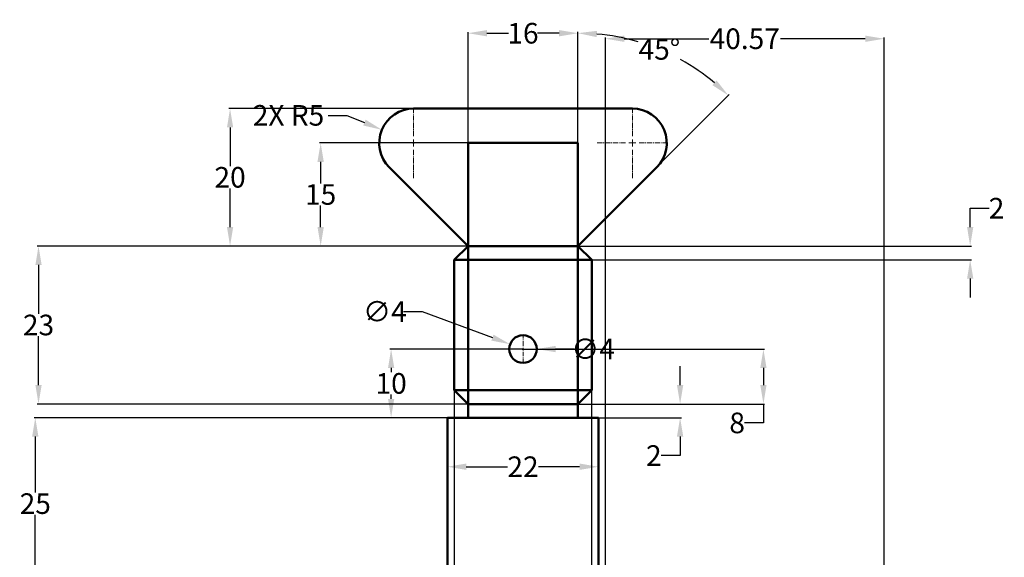
# Model space of a CAD drawing. Units: inches. Extents: x 7239 to 7401, y 3529 to 3727.
# Tile 2 of 2: x 7258 to 7401, y 3648 to 3727. Entities that reach past the tile are written whole.
import ezdxf

# ---------------------------------------------------------------- set-up
doc = ezdxf.new("R2010")
doc.units = ezdxf.units.IN
doc.header["$MEASUREMENT"] = 0
doc.linetypes.add('CENTER2', pattern=[1.125, 0.75, -0.125, 0.125, -0.125])
for name, color, linetype, lineweight in [('M-CNTR', 4, 'CENTER2', 18), ('M-DIMS', 2, 'Continuous', 25), ('M-OUTL', 7, 'Continuous', 50)]:
    doc.layers.add(name, color=color, linetype=linetype, lineweight=lineweight)
doc.styles.get("Standard").update_dxf_attribs({"font": 'arial.ttf'})
doc.dimstyles.get("Standard").update_dxf_attribs({"dimtxt": 3, "dimasz": 2.75, "dimexe": 0.18, "dimexo": 0.0625, "dimgap": 0.09, "dimtad": 0, "dimtih": 1, "dimtoh": 1, "dimdec": 0, "dimzin": 0, "dimdsep": 46, "dimtxsty": 'Standard', "dimcen": 0.09, "dimadec": 0, "dimazin": 0, "dimtfac": 1, "dimtdec": 0, "dimtofl": 0, "dimtmove": 0, "dimatfit": 3, "dimfxl": 1, "dimtolj": 1, "dimtzin": 0, "dimarcsym": 0})

# ---------------------------------------------------------------- blocks, each defined once
blk = doc.blocks.new('*U2')
at = {"layer": 'M-CNTR', "color": 0, "transparency": 16777216}
for p, q in [((0, 1), (0, 5.12)), ((-5.12, 0), (-1, 0)), ((1, 0), (5.12, 0)), ((0, -5.12), (0, -1))]:
    blk.add_line(p, q, dxfattribs=at)
at = {"layer": 'M-CNTR', "color": 0, "linetype": 'Continuous', "transparency": 16777216}
for p, q in [((-0.5, 0), (0.5, 0)), ((0, -0.5), (0, 0.5))]:
    blk.add_line(p, q, dxfattribs=at)
blk = doc.blocks.new('*U3')
at = {"layer": 'M-CNTR', "color": 0, "transparency": 16777216}
for p, q in [((0, 1), (0, 5.12)), ((-5.12, 0), (-1, 0)), ((1, 0), (5.12, 0)), ((0, -5.12), (0, -1))]:
    blk.add_line(p, q, dxfattribs=at)
at = {"layer": 'M-CNTR', "color": 0, "linetype": 'Continuous', "transparency": 16777216}
for p, q in [((-0.5, 0), (0.5, 0)), ((0, -0.5), (0, 0.5))]:
    blk.add_line(p, q, dxfattribs=at)
blk = doc.blocks.new('*U4')
at = {"layer": 'M-CNTR', "color": 0, "transparency": 16777216}
for p, q in [((0, 0.4), (0, 2.12)), ((-2.12, 0), (-0.4, 0)), ((0.4, 0), (2.12, 0)), ((0, -2.12), (0, -0.4))]:
    blk.add_line(p, q, dxfattribs=at)
at = {"layer": 'M-CNTR', "color": 0, "linetype": 'Continuous', "transparency": 16777216}
for p, q in [((-0.2, 0), (0.2, 0)), ((0, -0.2), (0, 0.2))]:
    blk.add_line(p, q, dxfattribs=at)
blk = doc.blocks.new('*D21')
at = {"layer": 'Defpoints', "color": 0, "transparency": 16777216}
for p in [(7320.11, 3668.7), (7342.11, 3668.7), (7342.11, 3661.57)]:
    blk.add_point(p, dxfattribs=at)
at = {"layer": 'M-DIMS', "color": 0, "lineweight": -2, "transparency": 16777216}
for p, q in [((7320.11, 3668.64), (7320.11, 3661.39)), ((7342.11, 3668.64), (7342.11, 3661.39)), ((7322.86, 3661.57), (7328.87, 3661.57)), ((7339.36, 3661.57), (7333.36, 3661.57))]:
    blk.add_line(p, q, dxfattribs=at)
at = {"layer": 'M-DIMS', "color": 0, "transparency": 16777216}
for points in [[(7322.86, 3662.03), (7322.86, 3661.11), (7320.11, 3661.57)], [(7339.36, 3662.03), (7339.36, 3661.11), (7342.11, 3661.57)]]:
    blk.add_solid(points, dxfattribs=at)
at = {"layer": 'M-DIMS', "color": 0, "transparency": 16777216, "insert": (7331.11, 3661.57), "char_height": 3, "attachment_point": 5}
blk.add_mtext('\\A1;22', dxfattribs=at)
blk = doc.blocks.new('*D22')
at = {"layer": 'Defpoints', "color": 0, "transparency": 16777216}
for p in [(7260.1, 3668.7), (7320.11, 3668.7), (7320.11, 3643.7)]:
    blk.add_point(p, dxfattribs=at)
at = {"layer": 'M-DIMS', "color": 0, "lineweight": -2, "transparency": 16777216}
for p, q in [((7320.05, 3668.7), (7259.92, 3668.7)), ((7260.1, 3665.95), (7260.1, 3657.82)), ((7260.1, 3646.45), (7260.1, 3654.58)), ((7320.05, 3643.7), (7259.92, 3643.7))]:
    blk.add_line(p, q, dxfattribs=at)
at = {"layer": 'M-DIMS', "color": 0, "transparency": 16777216}
for points in [[(7259.64, 3665.95), (7260.56, 3665.95), (7260.1, 3668.7)], [(7259.64, 3646.45), (7260.56, 3646.45), (7260.1, 3643.7)]]:
    blk.add_solid(points, dxfattribs=at)
at = {"layer": 'M-DIMS', "color": 0, "transparency": 16777216, "insert": (7260.1, 3656.2), "char_height": 3, "attachment_point": 5}
blk.add_mtext('\\A1;25', dxfattribs=at)
blk = doc.blocks.new('*D23')
at = {"layer": 'Defpoints', "color": 0, "transparency": 16777216}
for p in [(7260.57, 3693.7), (7323.11, 3693.7), (7323.11, 3670.7)]:
    blk.add_point(p, dxfattribs=at)
at = {"layer": 'M-DIMS', "color": 0, "lineweight": -2, "transparency": 16777216}
for p, q in [((7323.05, 3693.7), (7260.39, 3693.7)), ((7260.57, 3690.95), (7260.57, 3683.82)), ((7260.57, 3673.45), (7260.57, 3680.58)), ((7323.05, 3670.7), (7260.39, 3670.7))]:
    blk.add_line(p, q, dxfattribs=at)
at = {"layer": 'M-DIMS', "color": 0, "transparency": 16777216}
for points in [[(7260.12, 3690.95), (7261.03, 3690.95), (7260.57, 3693.7)], [(7260.12, 3673.45), (7261.03, 3673.45), (7260.57, 3670.7)]]:
    blk.add_solid(points, dxfattribs=at)
at = {"layer": 'M-DIMS', "color": 0, "transparency": 16777216, "insert": (7260.57, 3682.2), "char_height": 3, "attachment_point": 5}
blk.add_mtext('\\A1;23', dxfattribs=at)
blk = doc.blocks.new('*D24')
at = {"layer": 'Defpoints', "color": 0, "transparency": 16777216}
for p in [(7339.11, 3670.7), (7339.11, 3668.7), (7353.99, 3668.7)]:
    blk.add_point(p, dxfattribs=at)
at = {"layer": 'M-DIMS', "color": 0, "lineweight": -2, "transparency": 16777216}
for p, q in [((7353.99, 3673.45), (7353.99, 3676.2)), ((7339.18, 3670.7), (7354.17, 3670.7)), ((7339.18, 3668.7), (7354.17, 3668.7)), ((7353.99, 3665.95), (7353.99, 3663.2)), ((7353.99, 3663.2), (7351.24, 3663.2))]:
    blk.add_line(p, q, dxfattribs=at)
at = {"layer": 'M-DIMS', "color": 0, "transparency": 16777216}
for points in [[(7353.53, 3673.45), (7354.45, 3673.45), (7353.99, 3670.7)], [(7353.53, 3665.95), (7354.45, 3665.95), (7353.99, 3668.7)]]:
    blk.add_solid(points, dxfattribs=at)
at = {"layer": 'M-DIMS', "color": 0, "transparency": 16777216, "insert": (7350.16, 3663.2), "char_height": 3, "attachment_point": 5}
blk.add_mtext('\\A1;2', dxfattribs=at)
blk = doc.blocks.new('*D25')
at = {"layer": 'Defpoints', "color": 0, "transparency": 16777216}
for p in [(7323.11, 3724.67), (7323.11, 3708.7), (7339.11, 3708.7)]:
    blk.add_point(p, dxfattribs=at)
at = {"layer": 'M-DIMS', "color": 0, "lineweight": -2, "transparency": 16777216}
for p, q in [((7323.11, 3708.76), (7323.11, 3724.85)), ((7325.86, 3724.67), (7329.02, 3724.67)), ((7336.36, 3724.67), (7333.21, 3724.67)), ((7339.11, 3708.76), (7339.11, 3724.85))]:
    blk.add_line(p, q, dxfattribs=at)
at = {"layer": 'M-DIMS', "color": 0, "transparency": 16777216}
for points in [[(7325.86, 3725.13), (7325.86, 3724.21), (7323.11, 3724.67)], [(7336.36, 3725.13), (7336.36, 3724.21), (7339.11, 3724.67)]]:
    blk.add_solid(points, dxfattribs=at)
at = {"layer": 'M-DIMS', "color": 0, "transparency": 16777216, "insert": (7331.11, 3724.67), "char_height": 3, "attachment_point": 5}
blk.add_mtext('\\A1;16', dxfattribs=at)
blk = doc.blocks.new('*D26')
at = {"layer": 'Defpoints', "color": 0, "transparency": 16777216}
for p in [(7301.65, 3708.7), (7323.11, 3708.7), (7323.11, 3693.7)]:
    blk.add_point(p, dxfattribs=at)
at = {"layer": 'M-DIMS', "color": 0, "lineweight": -2, "transparency": 16777216}
for p, q in [((7323.05, 3708.7), (7301.47, 3708.7)), ((7301.65, 3705.95), (7301.65, 3702.82)), ((7301.65, 3696.45), (7301.65, 3699.58)), ((7323.05, 3693.7), (7301.47, 3693.7))]:
    blk.add_line(p, q, dxfattribs=at)
at = {"layer": 'M-DIMS', "color": 0, "transparency": 16777216}
for points in [[(7301.19, 3705.95), (7302.11, 3705.95), (7301.65, 3708.7)], [(7301.19, 3696.45), (7302.11, 3696.45), (7301.65, 3693.7)]]:
    blk.add_solid(points, dxfattribs=at)
at = {"layer": 'M-DIMS', "color": 0, "transparency": 16777216, "insert": (7301.65, 3701.2), "char_height": 3, "attachment_point": 5}
blk.add_mtext('\\A1;15', dxfattribs=at)
blk = doc.blocks.new('*D27')
at = {"layer": 'Defpoints', "color": 0, "transparency": 16777216}
for p in [(7323.11, 3713.7), (7288.46, 3693.7), (7323.11, 3693.7)]:
    blk.add_point(p, dxfattribs=at)
at = {"layer": 'M-DIMS', "color": 0, "lineweight": -2, "transparency": 16777216}
for p, q in [((7323.05, 3713.7), (7288.28, 3713.7)), ((7288.46, 3710.95), (7288.46, 3705.32)), ((7288.46, 3696.45), (7288.46, 3702.08)), ((7323.05, 3693.7), (7288.28, 3693.7))]:
    blk.add_line(p, q, dxfattribs=at)
at = {"layer": 'M-DIMS', "color": 0, "transparency": 16777216}
for points in [[(7288.01, 3710.95), (7288.92, 3710.95), (7288.46, 3713.7)], [(7288.01, 3696.45), (7288.92, 3696.45), (7288.46, 3693.7)]]:
    blk.add_solid(points, dxfattribs=at)
at = {"layer": 'M-DIMS', "color": 0, "transparency": 16777216, "insert": (7288.46, 3703.7), "char_height": 3, "attachment_point": 5}
blk.add_mtext('\\A1;20', dxfattribs=at)
blk = doc.blocks.new('*D28')
at = {"layer": 'Defpoints', "color": 0, "transparency": 16777216}
for p in [(7329.24, 3679.4), (7332.99, 3678)]:
    blk.add_point(p, dxfattribs=at)
at = {"layer": 'M-DIMS', "color": 0, "lineweight": -2, "transparency": 16777216}
for p, q in [((7313.7, 3684.16), (7316.45, 3684.16)), ((7316.45, 3684.16), (7326.66, 3680.36)), ((7331.02, 3678.7), (7331.2, 3678.7)), ((7331.11, 3678.61), (7331.11, 3678.79))]:
    blk.add_line(p, q, dxfattribs=at)
at = {"layer": 'M-DIMS', "color": 0, "transparency": 16777216}
blk.add_solid([(7326.82, 3680.79), (7326.5, 3679.93), (7329.24, 3679.4)], dxfattribs=at)
at = {"layer": 'M-DIMS', "color": 0, "transparency": 16777216, "insert": (7311, 3684.16), "char_height": 3, "attachment_point": 5}
blk.add_mtext('\\A1;∅4', dxfattribs=at)
blk = doc.blocks.new('*D29')
at = {"layer": 'Defpoints', "color": 0, "transparency": 16777216}
for p in [(7331.02, 3678.7), (7331.02, 3670.7), (7366.12, 3670.7)]:
    blk.add_point(p, dxfattribs=at)
at = {"layer": 'M-DIMS', "color": 0, "lineweight": -2, "transparency": 16777216}
for p, q in [((7331.09, 3678.7), (7366.3, 3678.7)), ((7366.12, 3675.95), (7366.12, 3673.45)), ((7331.09, 3670.7), (7366.3, 3670.7)), ((7366.12, 3670.7), (7366.12, 3667.95)), ((7366.12, 3667.95), (7363.37, 3667.95))]:
    blk.add_line(p, q, dxfattribs=at)
at = {"layer": 'M-DIMS', "color": 0, "transparency": 16777216}
for points in [[(7365.66, 3675.95), (7366.57, 3675.95), (7366.12, 3678.7)], [(7365.66, 3673.45), (7366.57, 3673.45), (7366.12, 3670.7)]]:
    blk.add_solid(points, dxfattribs=at)
at = {"layer": 'M-DIMS', "color": 0, "transparency": 16777216, "insert": (7362.29, 3667.95), "char_height": 3, "attachment_point": 5}
blk.add_mtext('\\A1;8', dxfattribs=at)
blk = doc.blocks.new('*D30')
at = {"layer": 'Defpoints', "color": 0, "transparency": 16777216}
for p in [(7331.02, 3678.7), (7311.91, 3668.7), (7331.11, 3668.7)]:
    blk.add_point(p, dxfattribs=at)
at = {"layer": 'M-DIMS', "color": 0, "lineweight": -2, "transparency": 16777216}
for p, q in [((7330.96, 3678.7), (7311.73, 3678.7)), ((7311.91, 3675.95), (7311.91, 3675.32)), ((7311.91, 3671.45), (7311.91, 3672.08)), ((7331.05, 3668.7), (7311.73, 3668.7))]:
    blk.add_line(p, q, dxfattribs=at)
at = {"layer": 'M-DIMS', "color": 0, "transparency": 16777216}
for points in [[(7311.46, 3675.95), (7312.37, 3675.95), (7311.91, 3678.7)], [(7311.46, 3671.45), (7312.37, 3671.45), (7311.91, 3668.7)]]:
    blk.add_solid(points, dxfattribs=at)
at = {"layer": 'M-DIMS', "color": 0, "transparency": 16777216, "insert": (7311.91, 3673.7), "char_height": 3, "attachment_point": 5}
blk.add_mtext('\\A1;10', dxfattribs=at)
blk = doc.blocks.new('*D31')
at = {"layer": 'Defpoints', "color": 0, "transparency": 16777216}
for p in [(7354.6, 3720.53), (7339.11, 3708.7), (7350.58, 3705.16), (7339.11, 3693.7), (7339.11, 3693.7)]:
    blk.add_point(p, dxfattribs=at)
at = {"layer": 'M-DIMS', "color": 0, "lineweight": -2, "transparency": 16777216}
for p, q in [((7339.11, 3708.76), (7339.11, 3724.86)), ((7350.62, 3705.21), (7361.15, 3715.73))]:
    blk.add_line(p, q, dxfattribs=at)
for start, end in [(73.57, 84.9124), (50.0876, 61.1496)]:
    blk.add_arc((7339.11, 3693.7), 30.98, start, end, dxfattribs=at)
at = {"layer": 'M-DIMS', "color": 0, "transparency": 16777216}
for points in [[(7341.84, 3724.1), (7341.88, 3725.02), (7339.11, 3724.68)], [(7359.3, 3717.8), (7358.68, 3717.12), (7361.02, 3715.61)]]:
    blk.add_solid(points, dxfattribs=at)
at = {"layer": 'M-DIMS', "color": 0, "transparency": 16777216, "insert": (7350.97, 3722.32), "char_height": 3, "attachment_point": 5}
blk.add_mtext('\\A1;45°', dxfattribs=at)
blk = doc.blocks.new('*D33')
at = {"layer": 'Defpoints', "color": 0, "transparency": 16777216}
for p in [(7321.11, 3672.7), (7341.11, 3672.7), (7341.11, 3532.1)]:
    blk.add_point(p, dxfattribs=at)
at = {"layer": 'M-DIMS', "color": 0, "lineweight": -2, "transparency": 16777216}
for p, q in [((7321.11, 3672.64), (7321.11, 3531.92)), ((7341.11, 3672.64), (7341.11, 3531.92)), ((7323.86, 3532.1), (7328.85, 3532.1)), ((7338.36, 3532.1), (7333.37, 3532.1))]:
    blk.add_line(p, q, dxfattribs=at)
at = {"layer": 'M-DIMS', "color": 0, "transparency": 16777216}
for points in [[(7323.86, 3532.56), (7323.86, 3531.64), (7321.11, 3532.1)], [(7338.36, 3532.56), (7338.36, 3531.64), (7341.11, 3532.1)]]:
    blk.add_solid(points, dxfattribs=at)
at = {"layer": 'M-DIMS', "color": 0, "transparency": 16777216, "insert": (7331.11, 3532.1), "char_height": 3, "attachment_point": 5}
blk.add_mtext('\\A1;20', dxfattribs=at)
blk = doc.blocks.new('*D34')
at = {"layer": 'Defpoints', "color": 0, "transparency": 16777216}
for p in [(7339.11, 3693.7), (7396.22, 3693.7), (7341.11, 3691.7)]:
    blk.add_point(p, dxfattribs=at)
at = {"layer": 'M-DIMS', "color": 0, "lineweight": -2, "transparency": 16777216}
for p, q in [((7396.22, 3696.45), (7396.22, 3699.2)), ((7396.22, 3699.2), (7398.97, 3699.2)), ((7339.18, 3693.7), (7396.4, 3693.7)), ((7341.18, 3691.7), (7396.4, 3691.7)), ((7396.22, 3688.95), (7396.22, 3686.2))]:
    blk.add_line(p, q, dxfattribs=at)
at = {"layer": 'M-DIMS', "color": 0, "transparency": 16777216}
for points in [[(7395.77, 3696.45), (7396.68, 3696.45), (7396.22, 3693.7)], [(7395.77, 3688.95), (7396.68, 3688.95), (7396.22, 3691.7)]]:
    blk.add_solid(points, dxfattribs=at)
at = {"layer": 'M-DIMS', "color": 0, "transparency": 16777216, "insert": (7400.06, 3699.2), "char_height": 3, "attachment_point": 5}
blk.add_mtext('\\A1;2', dxfattribs=at)
blk = doc.blocks.new('*D35')
at = {"layer": 'Defpoints', "color": 0, "transparency": 16777216}
for p in [(7383.69, 3723.87), (7343.11, 3643.7), (7383.69, 3606.49)]:
    blk.add_point(p, dxfattribs=at)
at = {"layer": 'M-DIMS', "color": 0, "lineweight": -2, "transparency": 16777216}
for p, q in [((7343.11, 3643.76), (7343.11, 3724.05)), ((7345.86, 3723.87), (7358.19, 3723.87)), ((7380.94, 3723.87), (7368.61, 3723.87)), ((7383.69, 3606.55), (7383.69, 3724.05))]:
    blk.add_line(p, q, dxfattribs=at)
at = {"layer": 'M-DIMS', "color": 0, "transparency": 16777216}
for points in [[(7345.86, 3724.33), (7345.86, 3723.41), (7343.11, 3723.87)], [(7380.94, 3724.33), (7380.94, 3723.41), (7383.69, 3723.87)]]:
    blk.add_solid(points, dxfattribs=at)
at = {"layer": 'M-DIMS', "color": 0, "transparency": 16777216, "insert": (7363.4, 3723.87), "char_height": 3, "attachment_point": 5}
blk.add_mtext('\\A1;40.57', dxfattribs=at)
blk = doc.blocks.new('*D44')
at = {"layer": 'Defpoints', "color": 0, "transparency": 16777216}
for p in [(7310.57, 3710.61), (7315.19, 3708.7)]:
    blk.add_point(p, dxfattribs=at)
at = {"layer": 'M-DIMS', "color": 0, "lineweight": -2, "transparency": 16777216}
for p, q in [((7302.73, 3712.72), (7305.48, 3712.72)), ((7305.48, 3712.72), (7308.03, 3711.67)), ((7315.1, 3708.7), (7315.28, 3708.7)), ((7315.19, 3708.61), (7315.19, 3708.79))]:
    blk.add_line(p, q, dxfattribs=at)
at = {"layer": 'M-DIMS', "color": 0, "transparency": 16777216}
blk.add_solid([(7308.2, 3712.09), (7307.85, 3711.24), (7310.57, 3710.61)], dxfattribs=at)
at = {"layer": 'M-DIMS', "color": 0, "transparency": 16777216, "insert": (7296.97, 3712.72), "char_height": 3, "attachment_point": 5}
blk.add_mtext('\\A1;2X R5', dxfattribs=at)
blk = doc.blocks.new('*D46')
at = {"layer": 'Defpoints', "color": 0, "transparency": 16777216}
for p in [(7329.11, 3678.7), (7333.11, 3678.7)]:
    blk.add_point(p, dxfattribs=at)
at = {"layer": 'M-DIMS', "color": 0, "lineweight": -2, "transparency": 16777216}
for p, q in [((7331.02, 3678.7), (7331.2, 3678.7)), ((7331.11, 3678.61), (7331.11, 3678.79)), ((7338.61, 3678.7), (7335.86, 3678.7))]:
    blk.add_line(p, q, dxfattribs=at)
at = {"layer": 'M-DIMS', "color": 0, "transparency": 16777216}
blk.add_solid([(7335.86, 3679.16), (7335.86, 3678.24), (7333.11, 3678.7)], dxfattribs=at)
at = {"layer": 'M-DIMS', "color": 0, "transparency": 16777216, "insert": (7341.31, 3678.7), "char_height": 3, "attachment_point": 5}
blk.add_mtext('\\A1;∅4', dxfattribs=at)

msp = doc.modelspace()

# ---------------------------------------------------------------- linework, layer by layer
at = {"layer": 'M-OUTL'}
for p, q in [((7347.043, 3713.7), (7315.185, 3713.7)), ((7315.185, 3713.7), (7347.043, 3713.7)), ((7323.114, 3693.7), (7323.114, 3708.7)), ((7323.114, 3708.7), (7339.114, 3708.7)), ((7339.114, 3708.7), (7339.114, 3693.7)), ((7323.114, 3693.7), (7311.65, 3705.165)), ((7339.114, 3693.7), (7350.579, 3705.165)), ((7321.114, 3691.7), (7323.114, 3693.7)), ((7339.114, 3693.7), (7323.114, 3693.7)), ((7323.114, 3670.7), (7323.114, 3693.7)), ((7341.114, 3691.7), (7339.114, 3693.7)), ((7339.114, 3670.7), (7339.114, 3693.7)), ((7321.114, 3691.7), (7341.114, 3691.7)), ((7321.114, 3691.7), (7321.114, 3672.7)), ((7341.114, 3672.7), (7341.114, 3691.7)), ((7323.114, 3670.7), (7321.114, 3672.7)), ((7321.114, 3672.7), (7341.114, 3672.7)), ((7339.114, 3670.7), (7341.114, 3672.7)), ((7341.114, 3672.7), (7341.114, 3672.7)), ((7323.114, 3668.7), (7323.114, 3670.7)), ((7323.114, 3670.7), (7323.114, 3670.7)), ((7323.114, 3670.7), (7339.114, 3670.7)), ((7339.114, 3668.7), (7339.114, 3670.7)), ((7320.114, 3643.7), (7320.114, 3668.7)), ((7320.114, 3668.7), (7342.114, 3668.7)), ((7342.114, 3668.7), (7342.114, 3643.7))]:
    msp.add_line(p, q, dxfattribs=at)
msp.add_circle((7331.114, 3678.7), 2, dxfattribs=at)
for centre, start, end in [((7315.185, 3708.7), 90, 225), ((7347.043, 3708.7), 315, 90)]:
    msp.add_arc(centre, 5, start, end, dxfattribs=at)

# ---------------------------------------------------------------- block references
at = {"layer": 'M-CNTR'}
for name, p in [('*U3', (7315.185, 3708.7)), ('*U2', (7347.043, 3708.7)), ('*U4', (7331.114, 3678.7))]:
    msp.add_blockref(name, p, dxfattribs=at)

# ---------------------------------------------------------------- dimensions: what is measured, and where the dimension line sits
at = {"layer": 'M-DIMS'}
for p1, p2, distance, picture, middle in [((7339.114, 3708.7), (7323.114, 3708.7), -15.972, '*D25', (7331.114, 3724.672)), ((7323.114, 3693.7), (7323.114, 3708.7), 21.462, '*D26', (7301.652, 3701.2)), ((7323.114, 3670.7), (7323.114, 3693.7), 62.539, '*D23', (7260.575, 3682.2)), ((7339.114, 3670.7), (7339.114, 3668.7), 14.876, '*D24', (7350.156, 3663.2)), ((7320.114, 3643.7), (7320.114, 3668.7), 60.013, '*D22', (7260.101, 3656.2))]:
    dim = msp.add_aligned_dim(p1=p1, p2=p2, distance=distance, dimstyle='Standard', override={"dimclrd": 0, "dimclre": 0, "dimclrt": 0}, dxfattribs=at)
    dim.commit()
    dim.dimension.update_dxf_attribs({"geometry": picture, "text_midpoint": middle})
dim = msp.add_angular_dim_2l(base=(7354.604, 3720.53), line1=((7339.114, 3693.7), (7350.579, 3705.165)), line2=((7339.114, 3708.7), (7339.114, 3693.7)), dimstyle='Standard', override={"dimclrd": 0, "dimclre": 0, "dimclrt": 0}, dxfattribs=at)
dim.commit()
dim.dimension.update_dxf_attribs({"geometry": '*D31', "text_midpoint": (7350.97, 3722.322)})
for base, p1, p2, override, picture, middle in [((7383.685, 3723.87), (7343.114, 3643.7), (7383.685, 3606.492), {"dimdec": 2, "dimlfac": 1, "dimrnd": 0, "dimzin": 0, "dimdsep": 46, "dimlunit": 2}, '*D35', (7363.4, 3723.87)), ((7341.114, 3532.101), (7321.114, 3672.7), (7341.114, 3672.7), {"dimdec": 0, "dimlfac": 1, "dimrnd": 0, "dimzin": 0, "dimdsep": 46, "dimlunit": 2}, '*D33', (7331.114, 3532.101)), ((7342.114, 3661.568), (7320.114, 3668.7), (7342.114, 3668.7), {"dimclrd": 0, "dimclre": 0, "dimclrt": 0}, '*D21', (7331.114, 3661.568))]:
    dim = msp.add_linear_dim(base=base, p1=p1, p2=p2, dimstyle='Standard', override=override, dxfattribs=at)
    dim.commit()
    dim.dimension.update_dxf_attribs({"geometry": picture, "text_midpoint": middle})
dim = msp.add_radius_dim(center=(7315.185, 3708.7), mpoint=(7310.566, 3710.614), text='2X <>', dimstyle='Standard', override={"dimdec": 0, "dimlfac": 1, "dimrnd": 0, "dimzin": 0, "dimdsep": 46, "dimlunit": 2}, dxfattribs=at)
dim.commit()
dim.dimension.update_dxf_attribs({"geometry": '*D44', "text_midpoint": (7296.966, 3712.719)})
for base, p1, p2, override, picture, middle in [((7288.464, 3693.7), (7323.114, 3713.7), (7323.114, 3693.7), {"dimclrd": 0, "dimclre": 0, "dimclrt": 0}, '*D27', (7288.464, 3703.7)), ((7396.223, 3693.7), (7341.114, 3691.7), (7339.114, 3693.7), {"dimdec": 0, "dimlfac": 1, "dimrnd": 0, "dimzin": 0, "dimdsep": 46, "dimlunit": 2}, '*D34', (7400.057, 3699.2)), ((7311.914, 3668.7), (7331.024, 3678.7), (7331.114, 3668.7), {"dimclrd": 0, "dimclre": 0, "dimclrt": 0}, '*D30', (7311.914, 3673.7)), ((7366.116, 3670.7), (7331.024, 3678.7), (7331.024, 3670.7), {"dimclrd": 0, "dimclre": 0, "dimclrt": 0}, '*D29', (7362.288, 3667.95))]:
    dim = msp.add_linear_dim(base=base, p1=p1, p2=p2, angle=90, dimstyle='Standard', override=override, dxfattribs=at)
    dim.commit()
    dim.dimension.update_dxf_attribs({"geometry": picture, "text_midpoint": middle})
for p1, p2, override, picture, middle in [((7332.988, 3678.003), (7329.24, 3679.398), {"dimclrd": 0, "dimclre": 0, "dimclrt": 0}, '*D28', (7310.997, 3684.159)), ((7329.114, 3678.7), (7333.114, 3678.7), {"dimdec": 0, "dimlfac": 1, "dimrnd": 0, "dimzin": 0, "dimdsep": 46, "dimlunit": 2}, '*D46', (7338.614, 3678.699))]:
    dim = msp.add_diameter_dim_2p(p1=p1, p2=p2, dimstyle='Standard', override=override, dxfattribs=at)
    dim.commit()
    dim.dimension.update_dxf_attribs({"geometry": picture, "text_midpoint": middle, "dimtype": 163})

doc.saveas('drawing.dxf')
